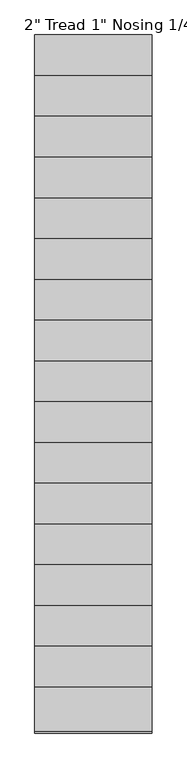
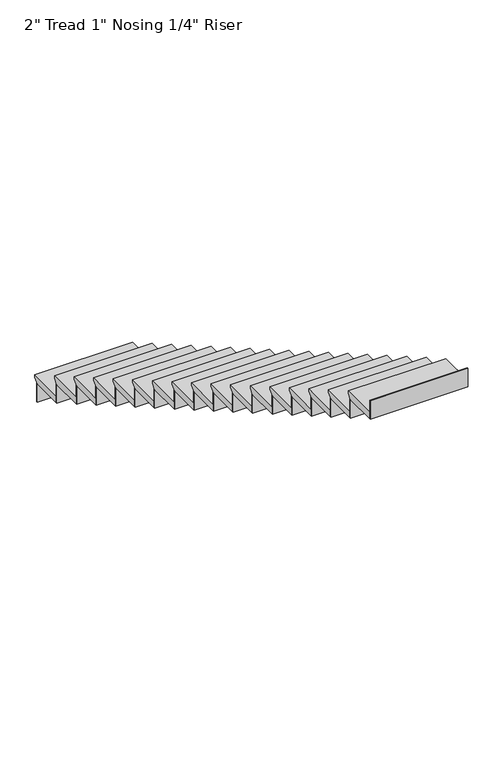
"""IFC4 building model written with IfcOpenShell, lengths in millimetres: stair flight geometry."""

from ifc_helpers import new_model, si_unit, frame, origin, place, context, project, spatial, polyline, outline, extrude, source, transform, mapped, element, save


def stair_flight_f2b89c93(model_context):
    return source(origin(), model_context, "Body", "SweptSolid", [
        extrude(outline(polyline([(5740.7076853, 4527.55), (6020.1076853, 4527.55), (6020.1076853, 4508.5), (5994.7076853, 4483.1), (5994.7076853, 4476.75), (5740.7076853, 4476.75), (5740.7076853, 4527.55)])), frame((-6854.5155596, 0.0, 0.0), z_axis=(1.0, 0.0, 0.0), x_axis=(0.0, 1.0, 0.0)), (0.0, 0.0, 1.0), 731.52),
        extrude(outline(polyline([(-6854.5155596, 5988.3576853), (-6854.5155596, 5994.7076853), (-6122.9955596, 5994.7076853), (-6122.9955596, 5988.3576853), (-6854.5155596, 5988.3576853)])), frame((0.0, 0.0, 4330.7), z_axis=(0.0, 0.0, 1.0), x_axis=(1.0, 0.0, 0.0)), (0.0, 0.0, 1.0), 146.05),
        extrude(outline(polyline([(-6854.5155596, 5734.3576853), (-6854.5155596, 5740.7076853), (-6122.9955596, 5740.7076853), (-6122.9955596, 5734.3576853), (-6854.5155596, 5734.3576853)])), frame((0.0, 0.0, 4476.75), z_axis=(0.0, 0.0, 1.0), x_axis=(1.0, 0.0, 0.0)), (0.0, 0.0, 1.0), 146.05),
        extrude(outline(polyline([(5486.7076853, 4673.6), (5766.1076853, 4673.6), (5766.1076853, 4654.55), (5740.7076853, 4629.15), (5740.7076853, 4622.8), (5486.7076853, 4622.8), (5486.7076853, 4673.6)])), frame((-6854.5155596, 0.0, 0.0), z_axis=(1.0, 0.0, 0.0), x_axis=(0.0, 1.0, 0.0)), (0.0, 0.0, 1.0), 731.52),
        extrude(outline(polyline([(-6854.5155596, 5480.3576853), (-6854.5155596, 5486.7076853), (-6122.9955596, 5486.7076853), (-6122.9955596, 5480.3576853), (-6854.5155596, 5480.3576853)])), frame((0.0, 0.0, 4622.8), z_axis=(0.0, 0.0, 1.0), x_axis=(1.0, 0.0, 0.0)), (0.0, 0.0, 1.0), 146.05),
        extrude(outline(polyline([(5232.7076853, 4819.65), (5512.1076853, 4819.65), (5512.1076853, 4800.6), (5486.7076853, 4775.2), (5486.7076853, 4768.85), (5232.7076853, 4768.85), (5232.7076853, 4819.65)])), frame((-6854.5155596, 0.0, 0.0), z_axis=(1.0, 0.0, 0.0), x_axis=(0.0, 1.0, 0.0)), (0.0, 0.0, 1.0), 731.52),
        extrude(outline(polyline([(-6854.5155596, 5226.3576853), (-6854.5155596, 5232.7076853), (-6122.9955596, 5232.7076853), (-6122.9955596, 5226.3576853), (-6854.5155596, 5226.3576853)])), frame((0.0, 0.0, 4768.85), z_axis=(0.0, 0.0, 1.0), x_axis=(1.0, 0.0, 0.0)), (0.0, 0.0, 1.0), 146.05),
        extrude(outline(polyline([(4978.7076853, 4965.7), (5258.1076853, 4965.7), (5258.1076853, 4946.65), (5232.7076853, 4921.25), (5232.7076853, 4914.9), (4978.7076853, 4914.9), (4978.7076853, 4965.7)])), frame((-6854.5155596, 0.0, 0.0), z_axis=(1.0, 0.0, 0.0), x_axis=(0.0, 1.0, 0.0)), (0.0, 0.0, 1.0), 731.52),
        extrude(outline(polyline([(-6854.5155596, 4972.3576853), (-6854.5155596, 4978.7076853), (-6122.9955596, 4978.7076853), (-6122.9955596, 4972.3576853), (-6854.5155596, 4972.3576853)])), frame((0.0, 0.0, 4914.9), z_axis=(0.0, 0.0, 1.0), x_axis=(1.0, 0.0, 0.0)), (0.0, 0.0, 1.0), 146.05),
        extrude(outline(polyline([(4724.7076853, 5111.75), (5004.1076853, 5111.75), (5004.1076853, 5092.7), (4978.7076853, 5067.3), (4978.7076853, 5060.95), (4724.7076853, 5060.95), (4724.7076853, 5111.75)])), frame((-6854.5155596, 0.0, 0.0), z_axis=(1.0, 0.0, 0.0), x_axis=(0.0, 1.0, 0.0)), (0.0, 0.0, 1.0), 731.52),
        extrude(outline(polyline([(-6854.5155596, 4718.3576853), (-6854.5155596, 4724.7076853), (-6122.9955596, 4724.7076853), (-6122.9955596, 4718.3576853), (-6854.5155596, 4718.3576853)])), frame((0.0, 0.0, 5060.95), z_axis=(0.0, 0.0, 1.0), x_axis=(1.0, 0.0, 0.0)), (0.0, 0.0, 1.0), 146.05),
        extrude(outline(polyline([(4470.7076853, 5257.8), (4750.1076853, 5257.8), (4750.1076853, 5238.75), (4724.7076853, 5213.35), (4724.7076853, 5207.0), (4470.7076853, 5207.0), (4470.7076853, 5257.8)])), frame((-6854.5155596, 0.0, 0.0), z_axis=(1.0, 0.0, 0.0), x_axis=(0.0, 1.0, 0.0)), (0.0, 0.0, 1.0), 731.52),
        extrude(outline(polyline([(-6854.5155596, 4464.3576853), (-6854.5155596, 4470.7076853), (-6122.9955596, 4470.7076853), (-6122.9955596, 4464.3576853), (-6854.5155596, 4464.3576853)])), frame((0.0, 0.0, 5207.0), z_axis=(0.0, 0.0, 1.0), x_axis=(1.0, 0.0, 0.0)), (0.0, 0.0, 1.0), 146.05),
        extrude(outline(polyline([(4216.7076853, 5403.85), (4496.1076853, 5403.85), (4496.1076853, 5384.8), (4470.7076853, 5359.4), (4470.7076853, 5353.05), (4216.7076853, 5353.05), (4216.7076853, 5403.85)])), frame((-6854.5155596, 0.0, 0.0), z_axis=(1.0, 0.0, 0.0), x_axis=(0.0, 1.0, 0.0)), (0.0, 0.0, 1.0), 731.52),
        extrude(outline(polyline([(-6854.5155596, 4210.3576853), (-6854.5155596, 4216.7076853), (-6122.9955596, 4216.7076853), (-6122.9955596, 4210.3576853), (-6854.5155596, 4210.3576853)])), frame((0.0, 0.0, 5353.05), z_axis=(0.0, 0.0, 1.0), x_axis=(1.0, 0.0, 0.0)), (0.0, 0.0, 1.0), 146.05),
        extrude(outline(polyline([(3962.7076853, 5549.9), (4242.1076853, 5549.9), (4242.1076853, 5530.85), (4216.7076853, 5505.45), (4216.7076853, 5499.1), (3962.7076853, 5499.1), (3962.7076853, 5549.9)])), frame((-6854.5155596, 0.0, 0.0), z_axis=(1.0, 0.0, 0.0), x_axis=(0.0, 1.0, 0.0)), (0.0, 0.0, 1.0), 731.52),
        extrude(outline(polyline([(-6854.5155596, 3956.3576853), (-6854.5155596, 3962.7076853), (-6122.9955596, 3962.7076853), (-6122.9955596, 3956.3576853), (-6854.5155596, 3956.3576853)])), frame((0.0, 0.0, 5499.1), z_axis=(0.0, 0.0, 1.0), x_axis=(1.0, 0.0, 0.0)), (0.0, 0.0, 1.0), 146.05),
        extrude(outline(polyline([(3708.7076853, 5695.95), (3988.1076853, 5695.95), (3988.1076853, 5676.9), (3962.7076853, 5651.5), (3962.7076853, 5645.15), (3708.7076853, 5645.15), (3708.7076853, 5695.95)])), frame((-6854.5155596, 0.0, 0.0), z_axis=(1.0, 0.0, 0.0), x_axis=(0.0, 1.0, 0.0)), (0.0, 0.0, 1.0), 731.52),
        extrude(outline(polyline([(-6854.5155596, 3702.3576853), (-6854.5155596, 3708.7076853), (-6122.9955596, 3708.7076853), (-6122.9955596, 3702.3576853), (-6854.5155596, 3702.3576853)])), frame((0.0, 0.0, 5645.15), z_axis=(0.0, 0.0, 1.0), x_axis=(1.0, 0.0, 0.0)), (0.0, 0.0, 1.0), 146.05),
        extrude(outline(polyline([(3454.7076853, 5842.0), (3734.1076853, 5842.0), (3734.1076853, 5822.95), (3708.7076853, 5797.55), (3708.7076853, 5791.2), (3454.7076853, 5791.2), (3454.7076853, 5842.0)])), frame((-6854.5155596, 0.0, 0.0), z_axis=(1.0, 0.0, 0.0), x_axis=(0.0, 1.0, 0.0)), (0.0, 0.0, 1.0), 731.52),
        extrude(outline(polyline([(-6854.5155596, 3448.3576853), (-6854.5155596, 3454.7076853), (-6122.9955596, 3454.7076853), (-6122.9955596, 3448.3576853), (-6854.5155596, 3448.3576853)])), frame((0.0, 0.0, 5791.2), z_axis=(0.0, 0.0, 1.0), x_axis=(1.0, 0.0, 0.0)), (0.0, 0.0, 1.0), 146.05),
        extrude(outline(polyline([(3200.7076853, 5988.05), (3480.1076853, 5988.05), (3480.1076853, 5969.0), (3454.7076853, 5943.6), (3454.7076853, 5937.25), (3200.7076853, 5937.25), (3200.7076853, 5988.05)])), frame((-6854.5155596, 0.0, 0.0), z_axis=(1.0, 0.0, 0.0), x_axis=(0.0, 1.0, 0.0)), (0.0, 0.0, 1.0), 731.52),
        extrude(outline(polyline([(-6854.5155596, 3194.3576853), (-6854.5155596, 3200.7076853), (-6122.9955596, 3200.7076853), (-6122.9955596, 3194.3576853), (-6854.5155596, 3194.3576853)])), frame((0.0, 0.0, 5937.25), z_axis=(0.0, 0.0, 1.0), x_axis=(1.0, 0.0, 0.0)), (0.0, 0.0, 1.0), 146.05),
        extrude(outline(polyline([(2946.7076853, 6134.1), (3226.1076853, 6134.1), (3226.1076853, 6115.05), (3200.7076853, 6089.65), (3200.7076853, 6083.3), (2946.7076853, 6083.3), (2946.7076853, 6134.1)])), frame((-6854.5155596, 0.0, 0.0), z_axis=(1.0, 0.0, 0.0), x_axis=(0.0, 1.0, 0.0)), (0.0, 0.0, 1.0), 731.52),
        extrude(outline(polyline([(-6854.5155596, 2940.3576853), (-6854.5155596, 2946.7076853), (-6122.9955596, 2946.7076853), (-6122.9955596, 2940.3576853), (-6854.5155596, 2940.3576853)])), frame((0.0, 0.0, 6083.3), z_axis=(0.0, 0.0, 1.0), x_axis=(1.0, 0.0, 0.0)), (0.0, 0.0, 1.0), 146.05),
        extrude(outline(polyline([(2692.7076853, 6280.15), (2972.1076853, 6280.15), (2972.1076853, 6261.1), (2946.7076853, 6235.7), (2946.7076853, 6229.35), (2692.7076853, 6229.35), (2692.7076853, 6280.15)])), frame((-6854.5155596, 0.0, 0.0), z_axis=(1.0, 0.0, 0.0), x_axis=(0.0, 1.0, 0.0)), (0.0, 0.0, 1.0), 731.52),
        extrude(outline(polyline([(-6854.5155596, 2686.3576853), (-6854.5155596, 2692.7076853), (-6122.9955596, 2692.7076853), (-6122.9955596, 2686.3576853), (-6854.5155596, 2686.3576853)])), frame((0.0, 0.0, 6229.35), z_axis=(0.0, 0.0, 1.0), x_axis=(1.0, 0.0, 0.0)), (0.0, 0.0, 1.0), 146.05),
        extrude(outline(polyline([(2438.7076853, 6426.2), (2718.1076853, 6426.2), (2718.1076853, 6407.15), (2692.7076853, 6381.75), (2692.7076853, 6375.4), (2438.7076853, 6375.4), (2438.7076853, 6426.2)])), frame((-6854.5155596, 0.0, 0.0), z_axis=(1.0, 0.0, 0.0), x_axis=(0.0, 1.0, 0.0)), (0.0, 0.0, 1.0), 731.52),
        extrude(outline(polyline([(-6854.5155596, 2432.3576853), (-6854.5155596, 2438.7076853), (-6122.9955596, 2438.7076853), (-6122.9955596, 2432.3576853), (-6854.5155596, 2432.3576853)])), frame((0.0, 0.0, 6375.4), z_axis=(0.0, 0.0, 1.0), x_axis=(1.0, 0.0, 0.0)), (0.0, 0.0, 1.0), 146.05),
        extrude(outline(polyline([(2184.7076853, 6572.25), (2464.1076853, 6572.25), (2464.1076853, 6553.2), (2438.7076853, 6527.8), (2438.7076853, 6521.45), (2184.7076853, 6521.45), (2184.7076853, 6572.25)])), frame((-6854.5155596, 0.0, 0.0), z_axis=(1.0, 0.0, 0.0), x_axis=(0.0, 1.0, 0.0)), (0.0, 0.0, 1.0), 731.52),
        extrude(outline(polyline([(-6854.5155596, 2178.3576853), (-6854.5155596, 2184.7076853), (-6122.9955596, 2184.7076853), (-6122.9955596, 2178.3576853), (-6854.5155596, 2178.3576853)])), frame((0.0, 0.0, 6521.45), z_axis=(0.0, 0.0, 1.0), x_axis=(1.0, 0.0, 0.0)), (0.0, 0.0, 1.0), 146.05),
        extrude(outline(polyline([(1930.7076853, 6718.3), (2210.1076853, 6718.3), (2210.1076853, 6699.25), (2184.7076853, 6673.85), (2184.7076853, 6667.5), (1930.7076853, 6667.5), (1930.7076853, 6718.3)])), frame((-6854.5155596, 0.0, 0.0), z_axis=(1.0, 0.0, 0.0), x_axis=(0.0, 1.0, 0.0)), (0.0, 0.0, 1.0), 731.52),
        extrude(outline(polyline([(-6854.5155596, 1924.3576853), (-6854.5155596, 1930.7076853), (-6122.9955596, 1930.7076853), (-6122.9955596, 1924.3576853), (-6854.5155596, 1924.3576853)])), frame((0.0, 0.0, 6667.5), z_axis=(0.0, 0.0, 1.0), x_axis=(1.0, 0.0, 0.0)), (0.0, 0.0, 1.0), 146.05),
        extrude(outline(polyline([(-6854.5155596, 1670.3576853), (-6854.5155596, 1676.7076853), (-6122.9955596, 1676.7076853), (-6122.9955596, 1670.3576853), (-6854.5155596, 1670.3576853)])), frame((0.0, 0.0, 6813.55), z_axis=(0.0, 0.0, 1.0), x_axis=(1.0, 0.0, 0.0)), (0.0, 0.0, 1.0), 146.05),
        extrude(outline(polyline([(1676.7076853, 6864.35), (1956.1076853, 6864.35), (1956.1076853, 6845.3), (1930.7076853, 6819.9), (1930.7076853, 6813.55), (1676.7076853, 6813.55), (1676.7076853, 6864.35)])), frame((-6854.5155596, 0.0, 0.0), z_axis=(1.0, 0.0, 0.0), x_axis=(0.0, 1.0, 0.0)), (0.0, 0.0, 1.0), 731.52),
    ])


if __name__ == "__main__":
    model = new_model("IFC4")
    model_context = context("Model", 3, world=origin())
    ifc_project = project(units=[si_unit("LENGTHUNIT", "METRE", prefix="MILLI")], contexts=[model_context])
    site = spatial("IfcSite", under=ifc_project)
    building = spatial("IfcBuilding", under=site)
    placement = place(None, origin())
    stair_flight_shape = stair_flight_f2b89c93(model_context)
    element("IfcStairFlight", 1, ObjectType="2\" Tread 1\" Nosing 1/4\" Riser", at=placement, inside=building, context=model_context, shape_type="MappedRepresentation", body=[
        mapped(stair_flight_shape, transform((0.0, 0.0, 0.0), x_axis=(1.0, 0.0, 0.0), y_axis=(0.0, 1.0, 0.0), z_axis=(0.0, 0.0, 1.0))),
    ])
    save(model, "model.ifc")
